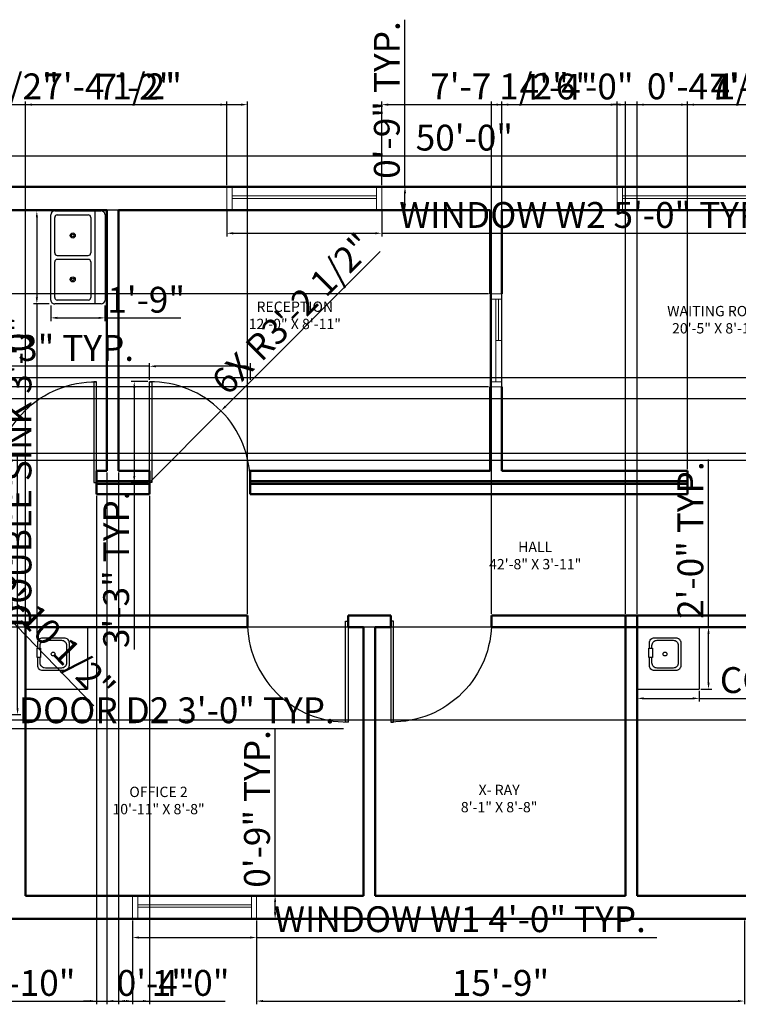
# Model space of a CAD drawing. Units: inches. Extents: x -53 to 650, y -41 to 348.
# Tile 2 of 3: x 131 to 410, y -33 to 348. Entities that reach past the tile are written whole.
import ezdxf

# ---------------------------------------------------------------- set-up
doc = ezdxf.new("R2010")
doc.units = ezdxf.units.IN
for name, color, linetype, lineweight in [('A-ANNO-DIMS', 2, 'Continuous', 18), ('A-AREA-IDEN', 7, 'Continuous', 25), ('A-DOOR', 3, 'Continuous', 25), ('A-FLOR-FIXT', 9, 'Continuous', 25), ('A-GLAZ', 4, 'Continuous', 18), ('A-WALL', 7, 'Continuous', 50), ('A-WALL-PATT', 7, 'Continuous', 13)]:
    doc.layers.add(name, color=color, linetype=linetype, lineweight=lineweight)
doc.styles.get("Standard").update_dxf_attribs({"font": 'arial.ttf'})
doc.dimstyles.new('ISO-25', dxfattribs={"dimtxt": 10, "dimasz": 2.5, "dimexe": 1.25, "dimexo": 0.625, "dimtad": 1, "dimlunit": 4, "dimtxsty": 'Standard', "dimcen": 2.5, "dimadec": 0, "dimazin": 0, "dimtfac": 1, "dimtmove": 0, "dimatfit": 3, "dimfxl": 1, "dimarcsym": 0})

# ---------------------------------------------------------------- blocks, each defined once
blk = doc.blocks.new('Sink-double - 36 in top')
for p, q in [((-18, -4), (18, -4)), ((-0.75, -18.5), (-0.75, -6.5)), ((0.75, -6.5), (0.75, -18.5))]:
    blk.add_line(p, q)
for points in [[(-16.5, 0), (16.5, 0)], [(-18, -19.5), (-18, -1.5)], [(18, -1.5), (18, -19.5)], [(-16.5, -18.5), (-16.5, -6.5)], [(-15.5, -5.5), (-1.75, -5.5)], [(1.75, -5.5), (15.5, -5.5)], [(16.5, -6.5), (16.5, -18.5)], [(16.5, -21), (-16.5, -21)], [(-1.75, -19.5), (-15.5, -19.5)], [(15.5, -19.5), (1.75, -19.5)]]:
    blk.add_lwpolyline(points)
for centre, radius in [((-8.5, -12.5), 1), ((-8.5, -12.5), 0.5), ((8.5, -12.5), 1), ((8.5, -12.5), 0.5)]:
    blk.add_circle(centre, radius)
for centre, radius, start, end in [((-16.5, -1.5), 1.5, 90, 180), ((16.5, -1.5), 1.5, 0, 90), ((-15.5, -6.5), 1, 90, 180), ((-1.75, -6.5), 1, 0, 90), ((1.75, -6.5), 1, 90, 180), ((15.5, -6.5), 1, 0, 90), ((-15.5, -18.5), 1, 180, 270), ((-1.75, -18.5), 1, 270, 0), ((1.75, -18.5), 1, 180, 270), ((15.5, -18.5), 1, 270, 0), ((-16.5, -19.5), 1.5, 180, 270), ((16.5, -19.5), 1.5, 270, 0)]:
    blk.add_arc(centre, radius, start, end)
blk = doc.blocks.new('*D4')
at = {"layer": 'A-ANNO-DIMS', "color": 0, "lineweight": -2, "transparency": 16777216}
for p, q in [((0, 284.12), (0, 296.76)), ((2.5, 295.51), (604.5, 295.51)), ((607, 284.12), (607, 296.76))]:
    blk.add_line(p, q, dxfattribs=at)
at = {"layer": 'A-ANNO-DIMS', "color": 0, "transparency": 16777216}
for points in [[(2.5, 295.92), (2.5, 295.09), (0, 295.51)], [(604.5, 295.92), (604.5, 295.09), (607, 295.51)]]:
    blk.add_solid(points, dxfattribs=at)
at = {"layer": 'Defpoints', "color": 0, "transparency": 16777216}
for p in [(607, 295.51), (0, 283.5), (607, 283.5)]:
    blk.add_point(p, dxfattribs=at)
at = {"layer": 'A-ANNO-DIMS', "color": 0, "transparency": 16777216, "insert": (303.5, 301.24), "char_height": 10, "attachment_point": 5}
blk.add_mtext('50\'-0"', dxfattribs=at)
blk = doc.blocks.new('DOOR-SWING-39IN')
for p, q in [((38, 0), (38, 39)), ((38, 39), (39, 39)), ((39, 39), (39, 0)), ((39, 0), (38, 0))]:
    blk.add_line(p, q)
blk.add_arc((38.5, 38.5), 38.5, 179.2559, 270.7441)
blk = doc.blocks.new('WIN-48IN')
for p, q in [((0, 9), (0, 0)), ((2, 0), (2, 9)), ((46, 0), (46, 9)), ((48, 9), (48, 0)), ((2, 5.5), (46, 5.5)), ((2, 4.5), (46, 4.5))]:
    blk.add_line(p, q)
blk.add_lwpolyline([(48, 9), (0, 9), (0, 0), (48, 0)], close=True)
blk = doc.blocks.new('WIN-60IN')
for p, q in [((0, 9), (0, 0)), ((2, 0), (2, 9)), ((58, 0), (58, 9)), ((60, 9), (60, 0)), ((2, 5.5), (58, 5.5)), ((2, 4.5), (58, 4.5))]:
    blk.add_line(p, q)
blk.add_lwpolyline([(60, 9), (0, 9), (0, 0), (60, 0)], close=True)
blk = doc.blocks.new('SINK-CORNER-24IN')
for p in [(24, 24), (0, 0)]:
    blk.add_line(p, (24, 0))
for points in [[(4.72, 15.9), (4.72, 17.89, -0.414214), (6.72, 19.89), (14.88, 19.89, -0.414214), (16.88, 17.89), (16.88, 9.16, -0.414214), (14.88, 7.16), (6.72, 7.16, -0.414214), (4.72, 9.16), (4.72, 12.24)], [(5.69, 15.9), (5.69, 16.92, -0.414214), (7.69, 18.92), (13.9, 18.92, -0.414214), (15.9, 16.92), (15.9, 10.14, -0.414214), (13.9, 8.14), (7.69, 8.14, -0.414214), (5.69, 10.14), (5.69, 12.24)]]:
    blk.add_lwpolyline(points, format="xyb")
blk.add_lwpolyline([(4.49, 15.9), (5.85, 15.9), (5.85, 12.24), (4.49, 12.24)], close=True)
blk.add_circle((10.73, 13.57), 0.751)
blk = doc.blocks.new('*D11')
at = {"layer": 'A-ANNO-DIMS', "color": 0, "lineweight": -2, "transparency": 16777216}
for p, q in [((181.5, 214.01), (49.76, 214.01)), ((181.5, 208.76), (181.5, 215.26)), ((218.13, 214.01), (184, 214.01)), ((220.63, 208.76), (220.63, 215.26))]:
    blk.add_line(p, q, dxfattribs=at)
at = {"layer": 'A-ANNO-DIMS', "color": 0, "transparency": 16777216}
for points in [[(184, 214.42), (184, 213.59), (181.5, 214.01)], [(218.13, 214.42), (218.13, 213.59), (220.63, 214.01)]]:
    blk.add_solid(points, dxfattribs=at)
at = {"layer": 'Defpoints', "color": 0, "transparency": 16777216}
for p in [(181.5, 214.01), (181.5, 208.13), (220.63, 208.13)]:
    blk.add_point(p, dxfattribs=at)
at = {"layer": 'A-ANNO-DIMS', "color": 0, "transparency": 16777216, "insert": (114.38, 219.81), "char_height": 10, "attachment_point": 5}
blk.add_mtext('DOOR D1 3\'-3" TYP.', dxfattribs=at)
blk = doc.blocks.new('*D12')
at = {"layer": 'A-ANNO-DIMS', "color": 0, "lineweight": -2, "transparency": 16777216}
for p, q in [((180.88, 208.13), (174.38, 208.13)), ((175.63, 205.63), (175.63, 171.5)), ((180.88, 169), (174.38, 169)), ((175.63, 169), (175.63, 104.3))]:
    blk.add_line(p, q, dxfattribs=at)
at = {"layer": 'A-ANNO-DIMS', "color": 0, "transparency": 16777216}
for points in [[(175.21, 205.63), (176.05, 205.63), (175.63, 208.13)], [(175.21, 171.5), (176.05, 171.5), (175.63, 169)]]:
    blk.add_solid(points, dxfattribs=at)
at = {"layer": 'Defpoints', "color": 0, "transparency": 16777216}
for p in [(181.5, 208.13), (175.63, 169), (181.5, 169)]:
    blk.add_point(p, dxfattribs=at)
at = {"layer": 'A-ANNO-DIMS', "color": 0, "transparency": 16777216, "insert": (169.9, 135.4), "char_height": 10, "attachment_point": 5, "rotation": 90}
blk.add_mtext('3\'-3" TYP.', dxfattribs=at)
blk = doc.blocks.new('*D13')
at = {"layer": 'A-ANNO-DIMS', "color": 0, "lineweight": -2, "transparency": 16777216}
for p, q in [((88.86, 78.49), (88.86, 72.44)), ((125, 78.49), (125, 72.44)), ((91.36, 73.69), (122.5, 73.69)), ((125, 73.69), (256.74, 73.69))]:
    blk.add_line(p, q, dxfattribs=at)
at = {"layer": 'A-ANNO-DIMS', "color": 0, "transparency": 16777216}
for points in [[(91.36, 74.11), (91.36, 73.28), (88.86, 73.69)], [(122.5, 74.11), (122.5, 73.28), (125, 73.69)]]:
    blk.add_solid(points, dxfattribs=at)
at = {"layer": 'Defpoints', "color": 0, "transparency": 16777216}
for p in [(88.86, 79.11), (125, 79.11), (125, 73.69)]:
    blk.add_point(p, dxfattribs=at)
at = {"layer": 'A-ANNO-DIMS', "color": 0, "transparency": 16777216, "insert": (192.12, 79.5), "char_height": 10, "attachment_point": 5}
blk.add_mtext('DOOR D2 3\'-0" TYP.', dxfattribs=at)
blk = doc.blocks.new('*D14')
at = {"layer": 'A-ANNO-DIMS', "color": 0, "lineweight": -2, "transparency": 16777216}
for p, q in [((130.42, 115.25), (130.42, 179.95)), ((125.62, 115.25), (131.67, 115.25)), ((130.42, 81.61), (130.42, 112.75)), ((125.62, 79.11), (131.67, 79.11))]:
    blk.add_line(p, q, dxfattribs=at)
at = {"layer": 'A-ANNO-DIMS', "color": 0, "transparency": 16777216}
for points in [[(130, 112.75), (130.84, 112.75), (130.42, 115.25)], [(130, 81.61), (130.84, 81.61), (130.42, 79.11)]]:
    blk.add_solid(points, dxfattribs=at)
at = {"layer": 'Defpoints', "color": 0, "transparency": 16777216}
for p in [(125, 115.25), (130.42, 115.25), (125, 79.11)]:
    blk.add_point(p, dxfattribs=at)
at = {"layer": 'A-ANNO-DIMS', "color": 0, "transparency": 16777216, "insert": (124.69, 148.85), "char_height": 10, "attachment_point": 5, "rotation": 90}
blk.add_mtext('3\'-0" TYP.', dxfattribs=at)
blk = doc.blocks.new('*D15')
at = {"layer": 'A-ANNO-DIMS', "color": 0, "lineweight": -2, "transparency": 16777216}
for p, q in [((175, -0.62), (175, -8.45)), ((223, -0.62), (223, -8.45)), ((177.5, -7.2), (220.5, -7.2)), ((223, -7.2), (378.13, -7.2))]:
    blk.add_line(p, q, dxfattribs=at)
at = {"layer": 'A-ANNO-DIMS', "color": 0, "transparency": 16777216}
for points in [[(177.5, -6.78), (177.5, -7.62), (175, -7.2)], [(220.5, -6.78), (220.5, -7.62), (223, -7.2)]]:
    blk.add_solid(points, dxfattribs=at)
at = {"layer": 'Defpoints', "color": 0, "transparency": 16777216}
for p in [(175, 0), (223, 0), (223, -7.2)]:
    blk.add_point(p, dxfattribs=at)
at = {"layer": 'A-ANNO-DIMS', "color": 0, "transparency": 16777216, "insert": (301.81, -1.4), "char_height": 10, "attachment_point": 5}
blk.add_mtext('WINDOW W1 4\'-0" TYP.', dxfattribs=at)
blk = doc.blocks.new('*D16')
at = {"layer": 'A-ANNO-DIMS', "color": 0, "lineweight": -2, "transparency": 16777216}
for p, q in [((230.2, 9), (230.2, 73.7)), ((223.63, 9), (231.45, 9)), ((230.2, 2.5), (230.2, 6.5)), ((223.63, 0), (231.45, 0))]:
    blk.add_line(p, q, dxfattribs=at)
at = {"layer": 'A-ANNO-DIMS', "color": 0, "transparency": 16777216}
for points in [[(229.78, 6.5), (230.62, 6.5), (230.2, 9)], [(229.78, 2.5), (230.62, 2.5), (230.2, 0)]]:
    blk.add_solid(points, dxfattribs=at)
at = {"layer": 'Defpoints', "color": 0, "transparency": 16777216}
for p in [(223, 9), (230.2, 9), (223, 0)]:
    blk.add_point(p, dxfattribs=at)
at = {"layer": 'A-ANNO-DIMS', "color": 0, "transparency": 16777216, "insert": (224.47, 42.6), "char_height": 10, "attachment_point": 5, "rotation": 90}
blk.add_mtext('0\'-9" TYP.', dxfattribs=at)
blk = doc.blocks.new('*D17')
at = {"layer": 'A-ANNO-DIMS', "color": 0, "lineweight": -2, "transparency": 16777216}
for p, q in [((211.5, 273.88), (211.5, 264.25)), ((271.5, 273.88), (271.5, 264.25)), ((214, 265.5), (269, 265.5)), ((271.5, 265.5), (426.63, 265.5))]:
    blk.add_line(p, q, dxfattribs=at)
at = {"layer": 'A-ANNO-DIMS', "color": 0, "transparency": 16777216}
for points in [[(214, 265.92), (214, 265.08), (211.5, 265.5)], [(269, 265.92), (269, 265.08), (271.5, 265.5)]]:
    blk.add_solid(points, dxfattribs=at)
at = {"layer": 'Defpoints', "color": 0, "transparency": 16777216}
for p in [(211.5, 274.5), (271.5, 274.5), (271.5, 265.5)]:
    blk.add_point(p, dxfattribs=at)
at = {"layer": 'A-ANNO-DIMS', "color": 0, "transparency": 16777216, "insert": (350.31, 271.3), "char_height": 10, "attachment_point": 5}
blk.add_mtext('WINDOW W2 5\'-0" TYP.', dxfattribs=at)
blk = doc.blocks.new('*D18')
at = {"layer": 'A-ANNO-DIMS', "color": 0, "lineweight": -2, "transparency": 16777216}
for p, q in [((280.5, 283.5), (280.5, 348.2)), ((272.13, 283.5), (281.75, 283.5)), ((280.5, 277), (280.5, 281)), ((272.13, 274.5), (281.75, 274.5))]:
    blk.add_line(p, q, dxfattribs=at)
at = {"layer": 'A-ANNO-DIMS', "color": 0, "transparency": 16777216}
for points in [[(280.08, 281), (280.92, 281), (280.5, 283.5)], [(280.08, 277), (280.92, 277), (280.5, 274.5)]]:
    blk.add_solid(points, dxfattribs=at)
at = {"layer": 'Defpoints', "color": 0, "transparency": 16777216}
for p in [(271.5, 283.5), (280.5, 283.5), (271.5, 274.5)]:
    blk.add_point(p, dxfattribs=at)
at = {"layer": 'A-ANNO-DIMS', "color": 0, "transparency": 16777216, "insert": (274.77, 317.1), "char_height": 10, "attachment_point": 5, "rotation": 90}
blk.add_mtext('0\'-9" TYP.', dxfattribs=at)
blk = doc.blocks.new('*D19')
at = {"layer": 'A-ANNO-DIMS', "color": 0, "lineweight": -2, "transparency": 16777216}
for p, q in [((370.5, 88.37), (370.5, 84.15)), ((394.5, 88.37), (394.5, 84.15)), ((373, 85.4), (392, 85.4)), ((394.5, 85.4), (560, 85.4))]:
    blk.add_line(p, q, dxfattribs=at)
at = {"layer": 'A-ANNO-DIMS', "color": 0, "transparency": 16777216}
for points in [[(373, 85.82), (373, 84.98), (370.5, 85.4)], [(392, 85.82), (392, 84.98), (394.5, 85.4)]]:
    blk.add_solid(points, dxfattribs=at)
at = {"layer": 'Defpoints', "color": 0, "transparency": 16777216}
for p in [(370.5, 89), (394.5, 89), (394.5, 85.4)]:
    blk.add_point(p, dxfattribs=at)
at = {"layer": 'A-ANNO-DIMS', "color": 0, "transparency": 16777216, "insert": (478.5, 91.2), "char_height": 10, "attachment_point": 5}
blk.add_mtext('CORNER SINK 2\'-0" TYP.', dxfattribs=at)
blk = doc.blocks.new('*D20')
at = {"layer": 'A-ANNO-DIMS', "color": 0, "lineweight": -2, "transparency": 16777216}
for p, q in [((398.1, 113), (398.1, 177.88)), ((395.13, 113), (399.35, 113)), ((398.1, 91.5), (398.1, 110.5)), ((395.13, 89), (399.35, 89))]:
    blk.add_line(p, q, dxfattribs=at)
at = {"layer": 'A-ANNO-DIMS', "color": 0, "transparency": 16777216}
for points in [[(397.68, 110.5), (398.52, 110.5), (398.1, 113)], [(397.68, 91.5), (398.52, 91.5), (398.1, 89)]]:
    blk.add_solid(points, dxfattribs=at)
at = {"layer": 'Defpoints', "color": 0, "transparency": 16777216}
for p in [(394.5, 113), (398.1, 113), (394.5, 89)]:
    blk.add_point(p, dxfattribs=at)
at = {"layer": 'A-ANNO-DIMS', "color": 0, "transparency": 16777216, "insert": (392.37, 146.69), "char_height": 10, "attachment_point": 5, "rotation": 90}
blk.add_mtext('2\'-0" TYP.', dxfattribs=at)
blk = doc.blocks.new('*D21')
at = {"layer": 'A-ANNO-DIMS', "color": 0, "lineweight": -2, "transparency": 16777216}
for p, q in [((142.68, 274.14), (136.65, 274.14)), ((137.9, 271.64), (137.9, 240.64)), ((142.68, 238.14), (136.65, 238.14)), ((137.9, 238.14), (137.9, 110.49))]:
    blk.add_line(p, q, dxfattribs=at)
at = {"layer": 'A-ANNO-DIMS', "color": 0, "transparency": 16777216}
for points in [[(137.49, 271.64), (138.32, 271.64), (137.9, 274.14)], [(137.49, 240.64), (138.32, 240.64), (137.9, 238.14)]]:
    blk.add_solid(points, dxfattribs=at)
at = {"layer": 'Defpoints', "color": 0, "transparency": 16777216}
for p in [(143.3, 274.14), (137.9, 238.14), (143.3, 238.14)]:
    blk.add_point(p, dxfattribs=at)
at = {"layer": 'A-ANNO-DIMS', "color": 0, "transparency": 16777216, "insert": (132.1, 173.07), "char_height": 10, "attachment_point": 5, "rotation": 90}
blk.add_mtext('DOUBLE SINK 3\'-0"', dxfattribs=at)
blk = doc.blocks.new('*D22')
at = {"layer": 'A-ANNO-DIMS', "color": 0, "lineweight": -2, "transparency": 16777216}
for p, q in [((143.3, 237.52), (143.3, 231.49)), ((164.3, 237.52), (164.3, 231.49)), ((145.8, 232.74), (161.8, 232.74)), ((164.3, 232.74), (193.7, 232.74))]:
    blk.add_line(p, q, dxfattribs=at)
at = {"layer": 'A-ANNO-DIMS', "color": 0, "transparency": 16777216}
for points in [[(145.8, 233.16), (145.8, 232.33), (143.3, 232.74)], [(161.8, 233.16), (161.8, 232.33), (164.3, 232.74)]]:
    blk.add_solid(points, dxfattribs=at)
at = {"layer": 'Defpoints', "color": 0, "transparency": 16777216}
for p in [(143.3, 238.14), (164.3, 238.14), (164.3, 232.74)]:
    blk.add_point(p, dxfattribs=at)
at = {"layer": 'A-ANNO-DIMS', "color": 0, "transparency": 16777216, "insert": (180.25, 238.47), "char_height": 10, "attachment_point": 5}
blk.add_mtext('1\'-9"', dxfattribs=at)
blk = doc.blocks.new('*D28')
at = {"layer": 'A-ANNO-DIMS', "color": 0, "lineweight": -2, "transparency": 16777216}
for p, q in [((123, 284.12), (123, 316.56)), ((211.5, 284.12), (211.5, 316.56)), ((125.5, 315.31), (209, 315.31))]:
    blk.add_line(p, q, dxfattribs=at)
at = {"layer": 'A-ANNO-DIMS', "color": 0, "transparency": 16777216}
for points in [[(125.5, 315.72), (125.5, 314.89), (123, 315.31)], [(209, 315.72), (209, 314.89), (211.5, 315.31)]]:
    blk.add_solid(points, dxfattribs=at)
at = {"layer": 'Defpoints', "color": 0, "transparency": 16777216}
for p in [(211.5, 315.31), (123, 283.5), (211.5, 283.5)]:
    blk.add_point(p, dxfattribs=at)
at = {"layer": 'A-ANNO-DIMS', "color": 0, "transparency": 16777216, "insert": (167.25, 321.1), "char_height": 10, "attachment_point": 5}
blk.add_mtext('7\'-4 1/2"', dxfattribs=at)
blk = doc.blocks.new('*D29')
at = {"layer": 'A-ANNO-DIMS', "color": 0, "lineweight": -2, "transparency": 16777216}
for p, q in [((271.5, 284.12), (271.5, 316.56)), ((362.75, 284.12), (362.75, 316.56)), ((274, 315.31), (360.25, 315.31))]:
    blk.add_line(p, q, dxfattribs=at)
at = {"layer": 'A-ANNO-DIMS', "color": 0, "transparency": 16777216}
for points in [[(274, 315.72), (274, 314.89), (271.5, 315.31)], [(360.25, 315.72), (360.25, 314.89), (362.75, 315.31)]]:
    blk.add_solid(points, dxfattribs=at)
at = {"layer": 'Defpoints', "color": 0, "transparency": 16777216}
for p in [(362.75, 315.31), (271.5, 283.5), (362.75, 283.5)]:
    blk.add_point(p, dxfattribs=at)
at = {"layer": 'A-ANNO-DIMS', "color": 0, "transparency": 16777216, "insert": (317.12, 321.1), "char_height": 10, "attachment_point": 5}
blk.add_mtext('7\'-7 1/2"', dxfattribs=at)
blk = doc.blocks.new('*D33')
at = {"layer": 'A-ANNO-DIMS', "color": 0, "lineweight": -2, "transparency": 16777216}
for p, q in [((93, -0.62), (93, -33.05)), ((175, -0.62), (175, -33.05)), ((95.5, -31.8), (172.5, -31.8))]:
    blk.add_line(p, q, dxfattribs=at)
at = {"layer": 'A-ANNO-DIMS', "color": 0, "transparency": 16777216}
for points in [[(95.5, -31.39), (95.5, -32.22), (93, -31.8)], [(172.5, -31.39), (172.5, -32.22), (175, -31.8)]]:
    blk.add_solid(points, dxfattribs=at)
at = {"layer": 'Defpoints', "color": 0, "transparency": 16777216}
for p in [(93, 0), (175, 0), (175, -31.8)]:
    blk.add_point(p, dxfattribs=at)
at = {"layer": 'A-ANNO-DIMS', "color": 0, "transparency": 16777216, "insert": (134, -26.07), "char_height": 10, "attachment_point": 5}
blk.add_mtext('6\'-10"', dxfattribs=at)
blk = doc.blocks.new('*D34')
at = {"layer": 'A-ANNO-DIMS', "color": 0, "lineweight": -2, "transparency": 16777216}
for p, q in [((223, -0.62), (223, -33.05)), ((412, -0.62), (412, -33.05)), ((225.5, -31.8), (409.5, -31.8))]:
    blk.add_line(p, q, dxfattribs=at)
at = {"layer": 'A-ANNO-DIMS', "color": 0, "transparency": 16777216}
for points in [[(225.5, -31.39), (225.5, -32.22), (223, -31.8)], [(409.5, -31.39), (409.5, -32.22), (412, -31.8)]]:
    blk.add_solid(points, dxfattribs=at)
at = {"layer": 'Defpoints', "color": 0, "transparency": 16777216}
for p in [(223, 0), (412, 0), (412, -31.8)]:
    blk.add_point(p, dxfattribs=at)
at = {"layer": 'A-ANNO-DIMS', "color": 0, "transparency": 16777216, "insert": (317.5, -26.07), "char_height": 10, "attachment_point": 5}
blk.add_mtext('15\'-9"', dxfattribs=at)
blk = doc.blocks.new('*D37')
at = {"layer": 'A-ANNO-DIMS', "color": 0, "lineweight": -2, "transparency": 16777216}
for p, q in [((318, 174.12), (318, 316.56)), ((390, 174.12), (390, 316.56)), ((320.5, 315.31), (387.5, 315.31))]:
    blk.add_line(p, q, dxfattribs=at)
at = {"layer": 'A-ANNO-DIMS', "color": 0, "transparency": 16777216}
for points in [[(320.5, 315.72), (320.5, 314.89), (318, 315.31)], [(387.5, 315.72), (387.5, 314.89), (390, 315.31)]]:
    blk.add_solid(points, dxfattribs=at)
at = {"layer": 'Defpoints', "color": 0, "transparency": 16777216}
for p in [(390, 315.31), (318, 173.5), (390, 173.5)]:
    blk.add_point(p, dxfattribs=at)
at = {"layer": 'A-ANNO-DIMS', "color": 0, "transparency": 16777216, "insert": (354, 321.04), "char_height": 10, "attachment_point": 5}
blk.add_mtext('6\'-0"', dxfattribs=at)
blk = doc.blocks.new('*D38')
at = {"layer": 'A-ANNO-DIMS', "color": 0, "lineweight": -2, "transparency": 16777216}
for p, q in [((390, 174.12), (390, 316.56)), ((438, 174.12), (438, 316.56)), ((392.5, 315.31), (435.5, 315.31))]:
    blk.add_line(p, q, dxfattribs=at)
at = {"layer": 'A-ANNO-DIMS', "color": 0, "transparency": 16777216}
for points in [[(392.5, 315.72), (392.5, 314.89), (390, 315.31)], [(435.5, 315.72), (435.5, 314.89), (438, 315.31)]]:
    blk.add_solid(points, dxfattribs=at)
at = {"layer": 'Defpoints', "color": 0, "transparency": 16777216}
for p in [(438, 315.31), (390, 173.5), (438, 173.5)]:
    blk.add_point(p, dxfattribs=at)
at = {"layer": 'A-ANNO-DIMS', "color": 0, "transparency": 16777216, "insert": (414, 321.04), "char_height": 10, "attachment_point": 5}
blk.add_mtext('4\'-0"', dxfattribs=at)
blk = doc.blocks.new('*D39')
at = {"layer": 'A-ANNO-DIMS', "color": 0, "lineweight": -2, "transparency": 16777216}
for p, q in [((312.88, 242), (-33.06, 242)), ((-31.81, 208.5), (-31.81, 239.5)), ((312.88, 206), (-33.06, 206))]:
    blk.add_line(p, q, dxfattribs=at)
at = {"layer": 'A-ANNO-DIMS', "color": 0, "transparency": 16777216}
for points in [[(-32.22, 239.5), (-31.39, 239.5), (-31.81, 242)], [(-32.22, 208.5), (-31.39, 208.5), (-31.81, 206)]]:
    blk.add_solid(points, dxfattribs=at)
at = {"layer": 'Defpoints', "color": 0, "transparency": 16777216}
for p in [(-31.81, 242), (313.5, 242), (313.5, 206)]:
    blk.add_point(p, dxfattribs=at)
at = {"layer": 'A-ANNO-DIMS', "color": 0, "transparency": 16777216, "insert": (-37.54, 224), "char_height": 10, "attachment_point": 5, "rotation": 90}
blk.add_mtext('3\'-0"', dxfattribs=at)
blk = doc.blocks.new('*D40')
at = {"layer": 'A-ANNO-DIMS', "color": 0, "lineweight": -2, "transparency": 16777216}
for p, q in [((-31.81, 274.5), (-31.81, 328.3)), ((312.88, 274.5), (-33.06, 274.5)), ((-31.81, 244.5), (-31.81, 272)), ((312.88, 242), (-33.06, 242))]:
    blk.add_line(p, q, dxfattribs=at)
at = {"layer": 'A-ANNO-DIMS', "color": 0, "transparency": 16777216}
for points in [[(-32.22, 272), (-31.39, 272), (-31.81, 274.5)], [(-32.22, 244.5), (-31.39, 244.5), (-31.81, 242)]]:
    blk.add_solid(points, dxfattribs=at)
at = {"layer": 'Defpoints', "color": 0, "transparency": 16777216}
for p in [(-31.81, 274.5), (313.5, 274.5), (313.5, 242)]:
    blk.add_point(p, dxfattribs=at)
at = {"layer": 'A-ANNO-DIMS', "color": 0, "transparency": 16777216, "insert": (-37.6, 302.65), "char_height": 10, "attachment_point": 5, "rotation": 90}
blk.add_mtext('2\'-8 1/2"', dxfattribs=at)
blk = doc.blocks.new('*D43')
at = {"layer": 'A-ANNO-DIMS', "color": 0, "lineweight": -2, "transparency": 16777216}
for p, q in [((505.38, 113), (-33.05, 113)), ((-31.81, 79.5), (-31.81, 110.5)), ((505.38, 77), (-33.05, 77))]:
    blk.add_line(p, q, dxfattribs=at)
at = {"layer": 'A-ANNO-DIMS', "color": 0, "transparency": 16777216}
for points in [[(-32.22, 110.5), (-31.39, 110.5), (-31.81, 113)], [(-32.22, 79.5), (-31.39, 79.5), (-31.81, 77)]]:
    blk.add_solid(points, dxfattribs=at)
at = {"layer": 'Defpoints', "color": 0, "transparency": 16777216}
for p in [(-31.81, 113), (506, 113), (506, 77)]:
    blk.add_point(p, dxfattribs=at)
at = {"layer": 'A-ANNO-DIMS', "color": 0, "transparency": 16777216, "insert": (-37.54, 95), "char_height": 10, "attachment_point": 5, "rotation": 90}
blk.add_mtext('3\'-0"', dxfattribs=at)
blk = doc.blocks.new('*D44')
at = {"layer": 'A-ANNO-DIMS', "color": 0, "lineweight": -2, "transparency": 16777216}
for p, q in [((133.5, 113.62), (133.5, 316.56)), ((219.5, 118.12), (219.5, 316.56)), ((136, 315.31), (217, 315.31))]:
    blk.add_line(p, q, dxfattribs=at)
at = {"layer": 'A-ANNO-DIMS', "color": 0, "transparency": 16777216}
for points in [[(136, 315.72), (136, 314.89), (133.5, 315.31)], [(217, 315.72), (217, 314.89), (219.5, 315.31)]]:
    blk.add_solid(points, dxfattribs=at)
at = {"layer": 'Defpoints', "color": 0, "transparency": 16777216}
for p in [(219.5, 315.31), (219.5, 117.5), (133.5, 113)]:
    blk.add_point(p, dxfattribs=at)
at = {"layer": 'A-ANNO-DIMS', "color": 0, "transparency": 16777216, "insert": (176.5, 320.95), "char_height": 10, "attachment_point": 5}
blk.add_mtext('7\'-2"', dxfattribs=at)
blk = doc.blocks.new('*D45')
at = {"layer": 'A-ANNO-DIMS', "color": 0, "lineweight": -2, "transparency": 16777216}
for p, q in [((314, 118.12), (314, 316.56)), ((366, 118.12), (366, 316.56)), ((316.5, 315.31), (363.5, 315.31))]:
    blk.add_line(p, q, dxfattribs=at)
at = {"layer": 'A-ANNO-DIMS', "color": 0, "transparency": 16777216}
for points in [[(316.5, 315.72), (316.5, 314.89), (314, 315.31)], [(363.5, 315.72), (363.5, 314.89), (366, 315.31)]]:
    blk.add_solid(points, dxfattribs=at)
at = {"layer": 'Defpoints', "color": 0, "transparency": 16777216}
for p in [(366, 315.31), (314, 117.5), (366, 117.5)]:
    blk.add_point(p, dxfattribs=at)
at = {"layer": 'A-ANNO-DIMS', "color": 0, "transparency": 16777216, "insert": (340, 320.93), "char_height": 10, "attachment_point": 5}
blk.add_mtext('4\'-4"', dxfattribs=at)
blk = doc.blocks.new('*D46')
at = {"layer": 'A-ANNO-DIMS', "color": 0, "lineweight": -2, "transparency": 16777216}
for p, q in [((370.5, 118.12), (370.5, 316.56)), ((456.5, 118.12), (456.5, 316.56)), ((373, 315.31), (454, 315.31))]:
    blk.add_line(p, q, dxfattribs=at)
at = {"layer": 'A-ANNO-DIMS', "color": 0, "transparency": 16777216}
for points in [[(373, 315.72), (373, 314.89), (370.5, 315.31)], [(454, 315.72), (454, 314.89), (456.5, 315.31)]]:
    blk.add_solid(points, dxfattribs=at)
at = {"layer": 'Defpoints', "color": 0, "transparency": 16777216}
for p in [(456.5, 315.31), (370.5, 117.5), (456.5, 117.5)]:
    blk.add_point(p, dxfattribs=at)
at = {"layer": 'A-ANNO-DIMS', "color": 0, "transparency": 16777216, "insert": (413.5, 320.95), "char_height": 10, "attachment_point": 5}
blk.add_mtext('7\'-2"', dxfattribs=at)
blk = doc.blocks.new('*D48')
at = {"layer": 'A-ANNO-DIMS', "color": 0, "lineweight": -2, "transparency": 16777216}
for p, q in [((85.5, 118.12), (85.5, 316.56)), ((89, 118.12), (89, 316.56)), ((83, 315.31), (80.5, 315.31)), ((85.5, 315.31), (89, 315.31)), ((91.5, 315.31), (145.13, 315.31))]:
    blk.add_line(p, q, dxfattribs=at)
at = {"layer": 'A-ANNO-DIMS', "color": 0, "transparency": 16777216}
for points in [[(83, 315.72), (83, 314.89), (85.5, 315.31)], [(91.5, 315.72), (91.5, 314.89), (89, 315.31)]]:
    blk.add_solid(points, dxfattribs=at)
at = {"layer": 'Defpoints', "color": 0, "transparency": 16777216}
for p in [(89, 315.31), (85.5, 117.5), (89, 117.5)]:
    blk.add_point(p, dxfattribs=at)
at = {"layer": 'A-ANNO-DIMS', "color": 0, "transparency": 16777216, "insert": (119.57, 321.1), "char_height": 10, "attachment_point": 5}
blk.add_mtext('0\'-3 1/2"', dxfattribs=at)
blk = doc.blocks.new('*D49')
at = {"layer": 'A-ANNO-DIMS', "color": 0, "lineweight": -2, "transparency": 16777216}
for p, q in [((165, 172.88), (165, -33.06)), ((161, 163.88), (161, -33.06)), ((158.5, -31.8), (156, -31.8)), ((161, -31.8), (165, -31.8)), ((167.5, -31.8), (197.83, -31.8))]:
    blk.add_line(p, q, dxfattribs=at)
at = {"layer": 'A-ANNO-DIMS', "color": 0, "transparency": 16777216}
for points in [[(158.5, -31.39), (158.5, -32.22), (161, -31.8)], [(167.5, -31.39), (167.5, -32.22), (165, -31.8)]]:
    blk.add_solid(points, dxfattribs=at)
at = {"layer": 'Defpoints', "color": 0, "transparency": 16777216}
for p in [(165, 173.5), (161, 164.5), (165, -31.8)]:
    blk.add_point(p, dxfattribs=at)
at = {"layer": 'A-ANNO-DIMS', "color": 0, "transparency": 16777216, "insert": (183.92, -26.07), "char_height": 10, "attachment_point": 5}
blk.add_mtext('0\'-4"', dxfattribs=at)
blk = doc.blocks.new('*D50')
at = {"layer": 'A-ANNO-DIMS', "color": 0, "lineweight": -2, "transparency": 16777216}
for p, q in [((169.5, 172.88), (169.5, -33.06)), ((181.5, 163.88), (181.5, -33.06)), ((172, -31.8), (179, -31.8)), ((181.5, -31.8), (210.89, -31.8))]:
    blk.add_line(p, q, dxfattribs=at)
at = {"layer": 'A-ANNO-DIMS', "color": 0, "transparency": 16777216}
for points in [[(172, -31.39), (172, -32.22), (169.5, -31.8)], [(179, -31.39), (179, -32.22), (181.5, -31.8)]]:
    blk.add_solid(points, dxfattribs=at)
at = {"layer": 'Defpoints', "color": 0, "transparency": 16777216}
for p in [(169.5, 173.5), (181.5, 164.5), (181.5, -31.8)]:
    blk.add_point(p, dxfattribs=at)
at = {"layer": 'A-ANNO-DIMS', "color": 0, "transparency": 16777216, "insert": (197.45, -26.07), "char_height": 10, "attachment_point": 5}
blk.add_mtext('1\'-0"', dxfattribs=at)
blk = doc.blocks.new('*D52')
at = {"layer": 'A-ANNO-DIMS', "color": 0, "lineweight": -2, "transparency": 16777216}
for p, q in [((562.88, 209.5), (-33.06, 209.5)), ((-31.81, 180), (-31.81, 207)), ((562.88, 177.5), (-33.06, 177.5))]:
    blk.add_line(p, q, dxfattribs=at)
at = {"layer": 'A-ANNO-DIMS', "color": 0, "transparency": 16777216}
for points in [[(-32.22, 207), (-31.39, 207), (-31.81, 209.5)], [(-32.22, 180), (-31.39, 180), (-31.81, 177.5)]]:
    blk.add_solid(points, dxfattribs=at)
at = {"layer": 'Defpoints', "color": 0, "transparency": 16777216}
for p in [(-31.81, 209.5), (563.5, 209.5), (563.5, 177.5)]:
    blk.add_point(p, dxfattribs=at)
at = {"layer": 'A-ANNO-DIMS', "color": 0, "transparency": 16777216, "insert": (-37.54, 193.5), "char_height": 10, "attachment_point": 5, "rotation": 90}
blk.add_mtext('2\'-8"', dxfattribs=at)
blk = doc.blocks.new('*D53')
at = {"layer": 'A-ANNO-DIMS', "color": 0, "lineweight": -2, "transparency": 16777216}
for p, q in [((366, 118.12), (366, 316.56)), ((370.5, 118.12), (370.5, 316.56)), ((363.5, 315.31), (361, 315.31)), ((366, 315.31), (370.5, 315.31)), ((373, 315.31), (426.63, 315.31))]:
    blk.add_line(p, q, dxfattribs=at)
at = {"layer": 'A-ANNO-DIMS', "color": 0, "transparency": 16777216}
for points in [[(363.5, 315.72), (363.5, 314.89), (366, 315.31)], [(373, 315.72), (373, 314.89), (370.5, 315.31)]]:
    blk.add_solid(points, dxfattribs=at)
at = {"layer": 'Defpoints', "color": 0, "transparency": 16777216}
for p in [(370.5, 315.31), (366, 117.5), (370.5, 117.5)]:
    blk.add_point(p, dxfattribs=at)
at = {"layer": 'A-ANNO-DIMS', "color": 0, "transparency": 16777216, "insert": (401.07, 321.1), "char_height": 10, "attachment_point": 5}
blk.add_mtext('0\'-4 1/2"', dxfattribs=at)
blk = doc.blocks.new('*D56')
at = {"layer": 'A-ANNO-DIMS', "color": 0, "lineweight": -2, "transparency": 16777216}
for p, q in [((-31.81, 201.42), (-31.81, 230.81)), ((570.47, 201.42), (-33.05, 201.42)), ((-31.81, 182.73), (-31.81, 198.92)), ((570.47, 180.23), (-33.05, 180.23))]:
    blk.add_line(p, q, dxfattribs=at)
at = {"layer": 'A-ANNO-DIMS', "color": 0, "transparency": 16777216}
for points in [[(-32.22, 198.92), (-31.39, 198.92), (-31.81, 201.42)], [(-32.22, 182.73), (-31.39, 182.73), (-31.81, 180.23)]]:
    blk.add_solid(points, dxfattribs=at)
at = {"layer": 'Defpoints', "color": 0, "transparency": 16777216}
for p in [(-31.81, 201.42), (571.1, 201.42), (571.1, 180.23)]:
    blk.add_point(p, dxfattribs=at)
at = {"layer": 'A-ANNO-DIMS', "color": 0, "transparency": 16777216, "insert": (-37.54, 217.37), "char_height": 10, "attachment_point": 5, "rotation": 90}
blk.add_mtext('1\'-9"', dxfattribs=at)
blk = doc.blocks.new('*D60')
at = {"layer": 'A-ANNO-DIMS', "color": 0, "lineweight": -2, "transparency": 16777216}
for p, q in [((84.72, 160), (108.79, 135.24)), ((160.01, 82.56), (110.54, 133.45))]:
    blk.add_line(p, q, dxfattribs=at)
at = {"layer": 'A-ANNO-DIMS', "color": 0, "transparency": 16777216}
blk.add_solid([(110.83, 133.74), (110.24, 133.16), (108.79, 135.24)], dxfattribs=at)
at = {"layer": 'Defpoints', "color": 0, "transparency": 16777216}
for p in [(84.72, 160), (108.79, 135.24)]:
    blk.add_point(p, dxfattribs=at)
at = {"layer": 'A-ANNO-DIMS', "color": 0, "transparency": 16777216, "insert": (140.3, 111.15), "char_height": 10, "attachment_point": 5, "rotation": 314.1925}
blk.add_mtext('R2\'-10 1/2"', dxfattribs=at)
blk = doc.blocks.new('*D62')
at = {"layer": 'A-ANNO-DIMS', "color": 0, "lineweight": -2, "transparency": 16777216}
for p, q in [((270.92, 258.42), (210.99, 198.49)), ((182, 169.5), (209.23, 196.73))]:
    blk.add_line(p, q, dxfattribs=at)
at = {"layer": 'A-ANNO-DIMS', "color": 0, "transparency": 16777216}
blk.add_solid([(210.7, 198.79), (211.29, 198.2), (209.23, 196.73)], dxfattribs=at)
at = {"layer": 'Defpoints', "color": 0, "transparency": 16777216}
for p in [(209.23, 196.73), (182, 169.5)]:
    blk.add_point(p, dxfattribs=at)
at = {"layer": 'A-ANNO-DIMS', "color": 0, "transparency": 16777216, "insert": (237.74, 233.44), "char_height": 10, "attachment_point": 5, "rotation": 45}
blk.add_mtext('6X R3\'-2 1/2"', dxfattribs=at)

msp = doc.modelspace()

# ---------------------------------------------------------------- hatches: boundary and pattern name
at = {"layer": 'A-WALL-PATT'}
h = msp.add_hatch(color=256, dxfattribs=at)
h.dxf.hatch_style = 1
h.paths.add_polyline_path([(9, 169.5), (9, 168.5), (122, 168.5), (122, 169, -0.0032466), (121.997, 169.5)])
h.paths.add_polyline_path([(161, 169.5), (161, 168.5), (181.5, 168.5), (181.5, 169.5)])
h.paths.add_polyline_path([(220.503, 169.5), (220.503, 168.5), (390, 168.5), (390, 169.5)])
h.paths.add_polyline_path([(598, 168.5), (598, 169.5), (438, 169.5), (438, 168.5)])

# ---------------------------------------------------------------- linework, layer by layer
at = {"layer": 'A-GLAZ'}
for p, q in [((313.5, 242), (318, 242)), ((318, 242), (318, 240)), ((318, 240), (313.5, 240)), ((315.75, 208), (315.75, 240)), ((316.75, 224), (316.75, 240)), ((318, 224), (315.75, 224)), ((318, 208), (313.5, 208)), ((313.5, 206), (318, 206))]:
    msp.add_line(p, q, dxfattribs=at)
msp.add_lwpolyline([(318, 242), (313.5, 242), (313.5, 206), (318, 206)], close=True, dxfattribs=at)
at = {"layer": 'A-WALL'}
for p, q in [((123, 283.5), (467.5, 283.5)), ((123, 274.5), (165, 274.5)), ((165, 274.5), (165, 173.5)), ((169.5, 274.5), (169.5, 173.5)), ((169.5, 274.5), (313.5, 274.5)), ((313.5, 274.5), (313.5, 242)), ((318, 274.5), (318, 242)), ((318, 274.5), (467.5, 274.5)), ((313.5, 206), (313.5, 173.5)), ((318, 206), (318, 173.5)), ((161, 173.5), (161, 164.5)), ((161, 173.5), (165, 173.5)), ((169.5, 173.5), (181.5, 173.5)), ((181.5, 173.5), (181.5, 164.5)), ((220.5, 173.5), (220.5, 164.5)), ((220.5, 173.5), (313.5, 173.5)), ((318, 173.5), (390, 173.5)), ((390, 173.5), (390, 164.5)), ((161, 169.5), (181.5, 169.5)), ((161, 168.5), (181.5, 168.5)), ((220.5, 169.5), (390, 169.5)), ((220.5, 168.5), (390, 168.5)), ((161, 164.5), (181.5, 164.5)), ((220.5, 164.5), (390, 164.5)), ((125, 117.5), (219.5, 117.5)), ((219.5, 117.5), (219.5, 113)), ((258.5, 117.5), (258.5, 113)), ((258.5, 117.5), (275, 117.5)), ((275, 117.5), (275, 113)), ((314, 117.5), (314, 113)), ((314, 117.5), (456.5, 117.5)), ((366, 117.5), (366, 9)), ((370.5, 117.5), (370.5, 9)), ((133.5, 113), (133.5, 9)), ((133.5, 113), (219.5, 113)), ((258.5, 113), (264.5, 113)), ((264.5, 113), (264.5, 9)), ((269, 113), (269, 9)), ((269, 113), (275, 113)), ((314, 113), (456.5, 113)), ((133.5, 9), (264.5, 9)), ((269, 9), (366, 9)), ((370.5, 9), (501.5, 9)), ((93, 0), (607, 0))]:
    msp.add_line(p, q, dxfattribs=at)
for points in [[(181.5, 169.5), (161, 169.5), (161, 168.5), (181.5, 168.5)], [(220.503, 169.5), (390, 169.5), (390, 168.5), (220.503, 168.5)]]:
    msp.add_lwpolyline(points, close=True, dxfattribs=at)

# ---------------------------------------------------------------- block references
at = {"layer": 'A-DOOR', "extrusion": (0, 0, -1), "zscale": -1, "rotation": 180}
msp.add_blockref('DOOR-SWING-39IN', (-122, 208), dxfattribs=at)
at = {"layer": 'A-DOOR', "rotation": 180}
msp.add_blockref('DOOR-SWING-39IN', (220.5, 208), dxfattribs=at)
at = {"layer": 'A-DOOR'}
msp.add_blockref('DOOR-SWING-39IN', (219.5, 76.25), dxfattribs=at)
at = {"layer": 'A-DOOR', "extrusion": (0, 0, -1), "zscale": -1}
msp.add_blockref('DOOR-SWING-39IN', (-314, 76.25), dxfattribs=at)
at = {"layer": 'A-FLOR-FIXT', "rotation": 270}
msp.add_blockref('Sink-double - 36 in top', (164.304, 256.142), dxfattribs=at)
at = {"layer": 'A-FLOR-FIXT'}
for p in [(133.5, 89), (370.5, 89)]:
    msp.add_blockref('SINK-CORNER-24IN', p, dxfattribs=at)
at = {"layer": 'A-GLAZ'}
for name, p in [('WIN-60IN', (211.5, 274.5)), ('WIN-60IN', (362.75, 274.5)), ('WIN-48IN', (175, 0))]:
    msp.add_blockref(name, p, dxfattribs=at)

# ---------------------------------------------------------------- texts
at = {"layer": 'A-AREA-IDEN', "char_height": 4, "attachment_point": 1}
for s, insert in [('\\pxqc;RECEPTION\\P12\'-0" X 8\'-11"', (205.064, 239.06)), ('\\pxqc;WAITING ROOM\\P20\'-5" X 8\'-11"', (369.063, 237.371)), ('\\pxqc;HALL\\P42\'-8" X 3\'-11"', (298.179, 146.048)), ('\\pxqc;OFFICE 2\\P10\'-11" X 8\'-8"', (152.27, 51.198)), ('\\pxqc;X- RAY\\P8\'-1" X 8\'-8"', (284.218, 51.96))]:
    msp.add_mtext_dynamic_manual_height_columns(s, width=65.53067, gutter_width=12.5, heights=[0], dxfattribs=dict(at, insert=insert))

# ---------------------------------------------------------------- dimensions: what is measured, and where the dimension line sits
at = {"layer": 'A-ANNO-DIMS'}
for base, p1, p2, angle, text, picture, middle in [((280.5, 283.5), (271.5, 274.5), (271.5, 283.5), 90, '<> TYP.', '*D18', (274.769, 317.102)), ((137.904, 238.142), (143.304, 274.142), (143.304, 238.142), 270, 'DOUBLE SINK <>', '*D21', (132.102, 173.066)), ((181.5, 214.005), (220.635, 208.135), (181.5, 208.135), 180, 'DOOR D1 <> TYP.', '*D11', (114.381, 219.807)), ((175.63, 169), (181.5, 208.135), (181.5, 169), 270, '<> TYP.', '*D12', (169.896, 135.401)), ((130.42, 115.25), (125, 79.115), (125, 115.25), 90, '<> TYP.', '*D14', (124.686, 148.849)), ((398.1, 113), (394.5, 89), (394.5, 113), 90, '<> TYP.', '*D20', (392.369, 146.688)), ((230.2, 9), (223, 0), (223, 9), 90, '<> TYP.', '*D16', (224.469, 42.602))]:
    dim = msp.add_linear_dim(base=base, p1=p1, p2=p2, angle=angle, text=text, dimstyle='ISO-25', override={"dimdec": 1, "dimlfac": 1, "dimrnd": 0, "dimzin": 1, "dimdsep": 46, "dimlunit": 4, "dimfrac": 2}, dxfattribs=at)
    dim.commit()
    dim.dimension.update_dxf_attribs({"geometry": picture, "text_midpoint": middle})
for base, p1, p2, picture, middle in [((89, 315.305), (85.5, 117.5), (89, 117.5), '*D48', (119.567, 321.104)), ((211.5, 315.305), (123, 283.5), (211.5, 283.5), '*D28', (167.25, 321.101)), ((362.75, 315.305), (271.5, 283.5), (362.75, 283.5), '*D29', (317.125, 321.10053206)), ((370.5, 315.305), (366, 117.5), (370.5, 117.5), '*D53', (401.067, 321.101)), ((219.5, 315.305), (133.5, 113), (219.5, 117.5), '*D44', (176.5, 320.95)), ((366, 315.305), (314, 117.5), (366, 117.5), '*D45', (340, 320.93)), ((390, 315.305), (318, 173.5), (390, 173.5), '*D37', (354, 321.036)), ((456.5, 315.305), (370.5, 117.5), (456.5, 117.5), '*D46', (413.5, 320.95)), ((438, 315.305), (390, 173.5), (438, 173.5), '*D38', (414, 321.036)), ((164.304, 232.742), (143.304, 238.142), (164.304, 238.142), '*D22', (180.25, 238.473)), ((165, -31.805), (161, 164.5), (165, 173.5), '*D49', (183.916, -26.074)), ((181.5, -31.805), (169.5, 173.5), (181.5, 164.5), '*D50', (197.446, -26.074)), ((175, -31.805), (93, 0), (175, 0), '*D33', (134, -26.074)), ((412, -31.805), (223, 0), (412, 0), '*D34', (317.5, -26.074))]:
    dim = msp.add_linear_dim(base=base, p1=p1, p2=p2, dimstyle='ISO-25', override={"dimdec": 1, "dimlfac": 1, "dimrnd": 0, "dimzin": 1, "dimdsep": 46, "dimlunit": 4, "dimfrac": 2}, dxfattribs=at)
    dim.commit()
    dim.dimension.update_dxf_attribs({"geometry": picture, "text_midpoint": middle})
for base, p1, p2, picture, middle in [((-31.805, 274.5), (313.5, 242), (313.5, 274.5), '*D40', (-37.601, 302.652)), ((-31.805, 242), (313.5, 206), (313.5, 242), '*D39', (-37.539, 224)), ((-31.805, 201.421), (571.095, 180.228), (571.095, 201.421), '*D56', (-37.536, 217.367)), ((-31.805, 209.5), (563.5, 177.5), (563.5, 209.5), '*D52', (-37.536, 193.5)), ((-31.805, 113), (506, 77), (506, 113), '*D43', (-37.539, 95))]:
    dim = msp.add_linear_dim(base=base, p1=p1, p2=p2, angle=90, dimstyle='ISO-25', override={"dimdec": 1, "dimlfac": 1, "dimrnd": 0, "dimzin": 1, "dimdsep": 46, "dimlunit": 4, "dimfrac": 2}, dxfattribs=at)
    dim.commit()
    dim.dimension.update_dxf_attribs({"geometry": picture, "text_midpoint": middle})
for base, p1, p2, text, override, picture, middle in [((607, 295.508), (0, 283.5), (607, 283.5), '50\'-0"', {"dimclrd": 0, "dimclre": 0, "dimclrt": 0}, '*D4', (303.5, 301.239)), ((271.5, 265.5), (211.5, 274.5), (271.5, 274.5), 'WINDOW W2 <> TYP.', {"dimdec": 1, "dimlfac": 1, "dimrnd": 0, "dimzin": 1, "dimdsep": 46, "dimlunit": 4, "dimfrac": 2}, '*D17', (350.314, 271.299)), ((394.5, 85.4), (370.5, 89), (394.5, 89), 'CORNER SINK <> TYP.', {"dimdec": 1, "dimlfac": 1, "dimrnd": 0, "dimzin": 1, "dimdsep": 46, "dimlunit": 4, "dimfrac": 2}, '*D19', (478.498, 91.199)), ((125, 73.695), (88.865, 79.115), (125, 79.115), 'DOOR D2 <> TYP.', {"dimdec": 1, "dimlfac": 1, "dimrnd": 0, "dimzin": 1, "dimdsep": 46, "dimlunit": 4, "dimfrac": 2}, '*D13', (192.119, 79.497)), ((223, -7.2), (175, 0), (223, 0), 'WINDOW W1 <> TYP.', {"dimdec": 1, "dimlfac": 1, "dimrnd": 0, "dimzin": 1, "dimdsep": 46, "dimlunit": 4, "dimfrac": 2}, '*D15', (301.814, -1.401))]:
    dim = msp.add_linear_dim(base=base, p1=p1, p2=p2, text=text, dimstyle='ISO-25', override=override, dxfattribs=at)
    dim.commit()
    dim.dimension.update_dxf_attribs({"geometry": picture, "text_midpoint": middle})
dim = msp.add_radius_dim(center=(182, 169.5), mpoint=(209.226, 196.726), text='6X <>', dimstyle='ISO-25', override={"dimdec": 1, "dimlfac": 1, "dimrnd": 0, "dimzin": 1, "dimdsep": 46, "dimlunit": 4, "dimfrac": 2}, dxfattribs=at)
dim.commit()
dim.dimension.update_dxf_attribs({"geometry": '*D62', "text_midpoint": (237.739, 233.44)})
dim = msp.add_radius_dim(center=(84.722, 160), mpoint=(108.793, 135.241), dimstyle='ISO-25', override={"dimdec": 1, "dimlfac": 1, "dimrnd": 0, "dimzin": 1, "dimdsep": 46, "dimlunit": 4, "dimfrac": 2}, dxfattribs=at)
dim.commit()
dim.dimension.update_dxf_attribs({"geometry": '*D60', "text_midpoint": (140.299, 111.148)})

doc.saveas('drawing.dxf')
